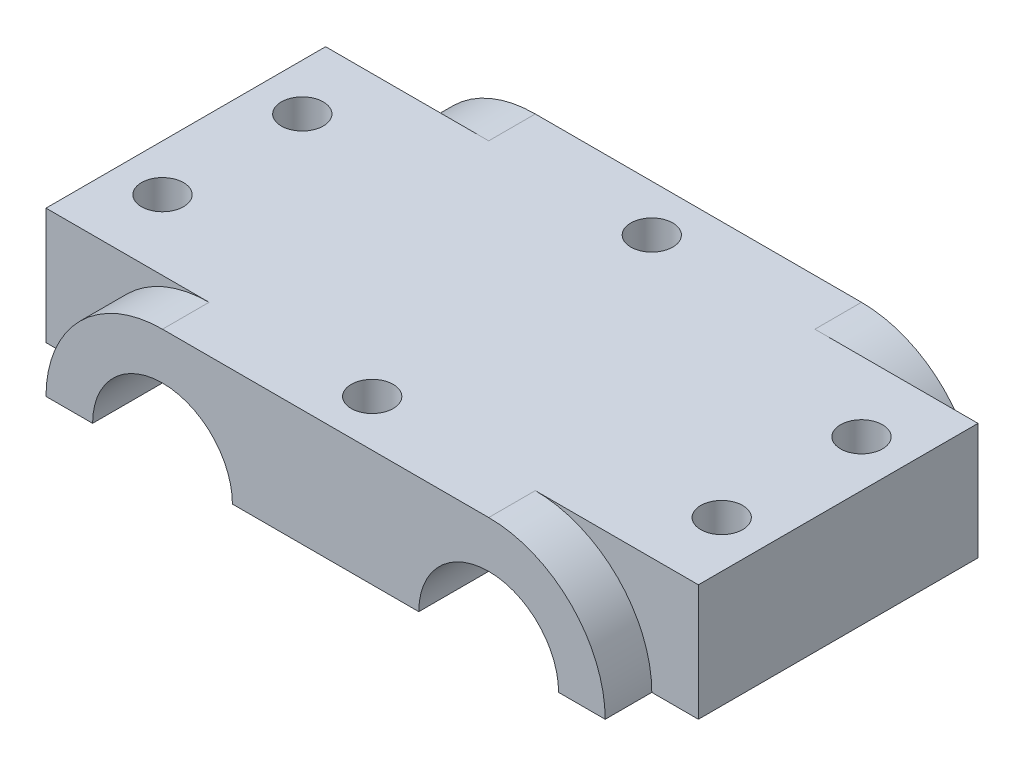
ISO-10303-21;
HEADER;
FILE_DESCRIPTION(('STEP AP214'),'2;1');
FILE_NAME('part.step','',(''),(''),'','','');
FILE_SCHEMA(('AUTOMOTIVE_DESIGN { 1 0 10303 214 1 1 1 1 }'));
ENDSEC;
DATA;
#1=APPLICATION_CONTEXT('core data for automotive mechanical design processes');
#2=APPLICATION_PROTOCOL_DEFINITION('international standard','automotive_design',2000,#1);
#3=PRODUCT_CONTEXT('',#1,'mechanical');
#4=PRODUCT('Part','Part','',(#3));
#5=PRODUCT_RELATED_PRODUCT_CATEGORY('part','',(#4));
#6=PRODUCT_DEFINITION_FORMATION('','',#4);
#7=PRODUCT_DEFINITION_CONTEXT('part definition',#1,'design');
#8=PRODUCT_DEFINITION('design','',#6,#7);
#9=PRODUCT_DEFINITION_SHAPE('','',#8);
#10=(LENGTH_UNIT() NAMED_UNIT(*) SI_UNIT(.MILLI.,.METRE.));
#11=(NAMED_UNIT(*) PLANE_ANGLE_UNIT() SI_UNIT($,.RADIAN.));
#12=(NAMED_UNIT(*) SI_UNIT($,.STERADIAN.) SOLID_ANGLE_UNIT());
#13=UNCERTAINTY_MEASURE_WITH_UNIT(LENGTH_MEASURE(1.E-05),#10,'distance_accuracy_value','');
#14=(GEOMETRIC_REPRESENTATION_CONTEXT(3) GLOBAL_UNCERTAINTY_ASSIGNED_CONTEXT((#13)) GLOBAL_UNIT_ASSIGNED_CONTEXT((#10,
#11,#12)) REPRESENTATION_CONTEXT('',''));
#15=CARTESIAN_POINT('',(0.,0.,0.));
#16=DIRECTION('',(0.,0.,1.));
#17=DIRECTION('',(1.,0.,0.));
#18=AXIS2_PLACEMENT_3D('',#15,#16,#17);
#19=CARTESIAN_POINT('',(35.,-6.25,20.));
#20=DIRECTION('',(0.,1.,0.));
#21=DIRECTION('',(-1.,0.,0.));
#22=AXIS2_PLACEMENT_3D('',#19,#20,#21);
#23=PLANE('',#22);
#24=CARTESIAN_POINT('',(0.,-6.25000000000001,-15.));
#25=DIRECTION('',(0.,1.,0.));
#26=DIRECTION('',(1.,0.,0.));
#27=AXIS2_PLACEMENT_3D('',#24,#25,#26);
#28=CIRCLE('',#27,2.25);
#29=CARTESIAN_POINT('',(2.25,-6.25000000000001,-15.));
#30=VERTEX_POINT('',#29);
#31=EDGE_CURVE('E271',#30,#30,#28,.T.);
#32=ORIENTED_EDGE('',*,*,#31,.T.);
#33=EDGE_LOOP('',(#32));
#34=FACE_BOUND('',#33,.T.);
#35=CARTESIAN_POINT('',(0.,-6.25000000000001,15.));
#36=DIRECTION('',(0.,1.,0.));
#37=DIRECTION('',(-1.,0.,0.));
#38=AXIS2_PLACEMENT_3D('',#35,#36,#37);
#39=CIRCLE('',#38,2.25);
#40=CARTESIAN_POINT('',(-2.24999999999999,-6.25000000000001,15.));
#41=VERTEX_POINT('',#40);
#42=EDGE_CURVE('E281',#41,#41,#39,.T.);
#43=ORIENTED_EDGE('',*,*,#42,.T.);
#44=EDGE_LOOP('',(#43));
#45=FACE_BOUND('',#44,.T.);
#46=DIRECTION('',(1.,0.,0.));
#47=VECTOR('',#46,1.);
#48=CARTESIAN_POINT('',(35.,-6.25,-20.));
#49=LINE('',#48,#47);
#50=CARTESIAN_POINT('',(-10.,-6.25,-20.));
#51=VERTEX_POINT('',#50);
#52=CARTESIAN_POINT('',(10.,-6.25,-20.));
#53=VERTEX_POINT('',#52);
#54=EDGE_CURVE('E158',#51,#53,#49,.T.);
#55=ORIENTED_EDGE('',*,*,#54,.T.);
#56=DIRECTION('',(0.,0.,1.));
#57=VECTOR('',#56,1.);
#58=CARTESIAN_POINT('',(10.,-6.25,-20.));
#59=LINE('',#58,#57);
#60=CARTESIAN_POINT('',(10.,-6.25,20.));
#61=VERTEX_POINT('',#60);
#62=EDGE_CURVE('E12',#53,#61,#59,.T.);
#63=ORIENTED_EDGE('',*,*,#62,.T.);
#64=DIRECTION('',(1.,0.,0.));
#65=VECTOR('',#64,1.);
#66=CARTESIAN_POINT('',(35.,-6.25,20.));
#67=LINE('',#66,#65);
#68=CARTESIAN_POINT('',(-10.,-6.25,20.));
#69=VERTEX_POINT('',#68);
#70=EDGE_CURVE('E177',#69,#61,#67,.T.);
#71=ORIENTED_EDGE('',*,*,#70,.F.);
#72=DIRECTION('',(0.,0.,1.));
#73=VECTOR('',#72,1.);
#74=CARTESIAN_POINT('',(-10.,-6.25,-20.));
#75=LINE('',#74,#73);
#76=EDGE_CURVE('E174',#51,#69,#75,.T.);
#77=ORIENTED_EDGE('',*,*,#76,.F.);
#78=EDGE_LOOP('',(#55,#63,#71,#77));
#79=FACE_BOUND('',#78,.T.);
#80=ADVANCED_FACE('F37',(#34,#45,#79),#23,.F.);
#81=CARTESIAN_POINT('',(35.,-33.75,-15.));
#82=DIRECTION('',(0.,0.,-1.));
#83=DIRECTION('',(-1.,0.,0.));
#84=AXIS2_PLACEMENT_3D('',#81,#82,#83);
#85=PLANE('',#84);
#86=DIRECTION('',(-1.,0.,0.));
#87=VECTOR('',#86,1.);
#88=CARTESIAN_POINT('',(35.,-6.25,-15.));
#89=LINE('',#88,#87);
#90=CARTESIAN_POINT('',(35.,-6.25,-15.));
#91=VERTEX_POINT('',#90);
#92=CARTESIAN_POINT('',(30.,-6.25,-15.));
#93=VERTEX_POINT('',#92);
#94=EDGE_CURVE('E180',#91,#93,#89,.T.);
#95=ORIENTED_EDGE('',*,*,#94,.T.);
#96=CARTESIAN_POINT('',(17.5,-6.25,-15.));
#97=DIRECTION('',(0.,0.,1.));
#98=DIRECTION('',(-1.,0.,0.));
#99=AXIS2_PLACEMENT_3D('',#96,#97,#98);
#100=CIRCLE('',#99,12.5);
#101=CARTESIAN_POINT('',(17.5,6.25,-15.));
#102=VERTEX_POINT('',#101);
#103=EDGE_CURVE('E335',#93,#102,#100,.T.);
#104=ORIENTED_EDGE('',*,*,#103,.T.);
#105=DIRECTION('',(-1.,0.,0.));
#106=VECTOR('',#105,1.);
#107=CARTESIAN_POINT('',(35.,6.25,-15.));
#108=LINE('',#107,#106);
#109=CARTESIAN_POINT('',(35.,6.25,-15.));
#110=VERTEX_POINT('',#109);
#111=EDGE_CURVE('E212',#110,#102,#108,.T.);
#112=ORIENTED_EDGE('',*,*,#111,.F.);
#113=DIRECTION('',(0.,1.,0.));
#114=VECTOR('',#113,1.);
#115=CARTESIAN_POINT('',(35.,-33.75,-15.));
#116=LINE('',#115,#114);
#117=EDGE_CURVE('E64',#91,#110,#116,.T.);
#118=ORIENTED_EDGE('',*,*,#117,.F.);
#119=EDGE_LOOP('',(#95,#104,#112,#118));
#120=FACE_BOUND('',#119,.T.);
#121=ADVANCED_FACE('F332',(#120),#85,.T.);
#122=CARTESIAN_POINT('',(22.5,-33.75,15.));
#123=DIRECTION('',(0.,0.,1.));
#124=DIRECTION('',(1.,0.,0.));
#125=AXIS2_PLACEMENT_3D('',#122,#123,#124);
#126=PLANE('',#125);
#127=CARTESIAN_POINT('',(17.5,-6.25,15.));
#128=DIRECTION('',(0.,0.,1.));
#129=DIRECTION('',(-1.,0.,0.));
#130=AXIS2_PLACEMENT_3D('',#127,#128,#129);
#131=CIRCLE('',#130,12.5);
#132=CARTESIAN_POINT('',(30.,-6.25,15.));
#133=VERTEX_POINT('',#132);
#134=CARTESIAN_POINT('',(17.5,6.25,15.));
#135=VERTEX_POINT('',#134);
#136=EDGE_CURVE('E343',#133,#135,#131,.T.);
#137=ORIENTED_EDGE('',*,*,#136,.F.);
#138=DIRECTION('',(1.,0.,0.));
#139=VECTOR('',#138,1.);
#140=CARTESIAN_POINT('',(35.,-6.25,15.));
#141=LINE('',#140,#139);
#142=CARTESIAN_POINT('',(35.,-6.25,15.));
#143=VERTEX_POINT('',#142);
#144=EDGE_CURVE('E181',#133,#143,#141,.T.);
#145=ORIENTED_EDGE('',*,*,#144,.T.);
#146=DIRECTION('',(0.,1.,0.));
#147=VECTOR('',#146,1.);
#148=CARTESIAN_POINT('',(35.,-33.75,15.));
#149=LINE('',#148,#147);
#150=CARTESIAN_POINT('',(35.,6.25,15.));
#151=VERTEX_POINT('',#150);
#152=EDGE_CURVE('E214',#143,#151,#149,.T.);
#153=ORIENTED_EDGE('',*,*,#152,.T.);
#154=DIRECTION('',(1.,0.,0.));
#155=VECTOR('',#154,1.);
#156=CARTESIAN_POINT('',(22.5,6.25,15.));
#157=LINE('',#156,#155);
#158=EDGE_CURVE('E213',#135,#151,#157,.T.);
#159=ORIENTED_EDGE('',*,*,#158,.F.);
#160=EDGE_LOOP('',(#137,#145,#153,#159));
#161=FACE_BOUND('',#160,.T.);
#162=ADVANCED_FACE('F317',(#161),#126,.T.);
#163=CARTESIAN_POINT('',(30.,-6.25000000000001,-7.50000000000001));
#164=DIRECTION('',(0.,1.,0.));
#165=DIRECTION('',(-1.,0.,0.));
#166=AXIS2_PLACEMENT_3D('',#163,#164,#165);
#167=CYLINDRICAL_SURFACE('',#166,2.25);
#168=CARTESIAN_POINT('',(30.,6.25,-7.50000000000001));
#169=DIRECTION('',(0.,1.,0.));
#170=DIRECTION('',(1.,0.,0.));
#171=AXIS2_PLACEMENT_3D('',#168,#169,#170);
#172=CIRCLE('',#171,2.25);
#173=CARTESIAN_POINT('',(32.25,6.25,-7.50000000000001));
#174=VERTEX_POINT('',#173);
#175=EDGE_CURVE('E274',#174,#174,#172,.T.);
#176=ORIENTED_EDGE('',*,*,#175,.T.);
#177=EDGE_LOOP('',(#176));
#178=FACE_BOUND('',#177,.T.);
#179=CARTESIAN_POINT('',(30.,-6.25000000000001,-7.50000000000001));
#180=DIRECTION('',(0.,1.,0.));
#181=DIRECTION('',(1.,0.,0.));
#182=AXIS2_PLACEMENT_3D('',#179,#180,#181);
#183=CIRCLE('',#182,2.25);
#184=CARTESIAN_POINT('',(32.25,-6.25000000000001,-7.50000000000001));
#185=VERTEX_POINT('',#184);
#186=EDGE_CURVE('E279',#185,#185,#183,.T.);
#187=ORIENTED_EDGE('',*,*,#186,.F.);
#188=EDGE_LOOP('',(#187));
#189=FACE_BOUND('',#188,.T.);
#190=ADVANCED_FACE('F402',(#178,#189),#167,.F.);
#191=CARTESIAN_POINT('',(30.,-6.25000000000001,7.49999999999999));
#192=DIRECTION('',(0.,1.,0.));
#193=DIRECTION('',(-1.,0.,0.));
#194=AXIS2_PLACEMENT_3D('',#191,#192,#193);
#195=CYLINDRICAL_SURFACE('',#194,2.25);
#196=CARTESIAN_POINT('',(30.,6.25,7.49999999999999));
#197=DIRECTION('',(0.,1.,0.));
#198=DIRECTION('',(1.,0.,0.));
#199=AXIS2_PLACEMENT_3D('',#196,#197,#198);
#200=CIRCLE('',#199,2.25);
#201=CARTESIAN_POINT('',(32.25,6.25,7.49999999999999));
#202=VERTEX_POINT('',#201);
#203=EDGE_CURVE('E294',#202,#202,#200,.T.);
#204=ORIENTED_EDGE('',*,*,#203,.T.);
#205=EDGE_LOOP('',(#204));
#206=FACE_BOUND('',#205,.T.);
#207=CARTESIAN_POINT('',(30.,-6.25000000000001,7.49999999999999));
#208=DIRECTION('',(0.,1.,0.));
#209=DIRECTION('',(1.,0.,0.));
#210=AXIS2_PLACEMENT_3D('',#207,#208,#209);
#211=CIRCLE('',#210,2.25);
#212=CARTESIAN_POINT('',(32.25,-6.25000000000001,7.49999999999999));
#213=VERTEX_POINT('',#212);
#214=EDGE_CURVE('E280',#213,#213,#211,.T.);
#215=ORIENTED_EDGE('',*,*,#214,.F.);
#216=EDGE_LOOP('',(#215));
#217=FACE_BOUND('',#216,.T.);
#218=ADVANCED_FACE('F396',(#206,#217),#195,.F.);
#219=CARTESIAN_POINT('',(35.,6.25,20.));
#220=DIRECTION('',(0.,-1.,0.));
#221=DIRECTION('',(1.,0.,0.));
#222=AXIS2_PLACEMENT_3D('',#219,#220,#221);
#223=PLANE('',#222);
#224=CARTESIAN_POINT('',(0.,6.25,-15.));
#225=DIRECTION('',(0.,1.,0.));
#226=DIRECTION('',(1.,0.,0.));
#227=AXIS2_PLACEMENT_3D('',#224,#225,#226);
#228=CIRCLE('',#227,2.25);
#229=CARTESIAN_POINT('',(2.25,6.25,-15.));
#230=VERTEX_POINT('',#229);
#231=EDGE_CURVE('E290',#230,#230,#228,.T.);
#232=ORIENTED_EDGE('',*,*,#231,.F.);
#233=EDGE_LOOP('',(#232));
#234=FACE_BOUND('',#233,.T.);
#235=CARTESIAN_POINT('',(0.,6.25,15.));
#236=DIRECTION('',(0.,1.,0.));
#237=DIRECTION('',(-1.,0.,0.));
#238=AXIS2_PLACEMENT_3D('',#235,#236,#237);
#239=CIRCLE('',#238,2.25);
#240=CARTESIAN_POINT('',(-2.25,6.25,15.));
#241=VERTEX_POINT('',#240);
#242=EDGE_CURVE('E282',#241,#241,#239,.T.);
#243=ORIENTED_EDGE('',*,*,#242,.F.);
#244=EDGE_LOOP('',(#243));
#245=FACE_BOUND('',#244,.T.);
#246=CARTESIAN_POINT('',(-30.,6.25,-7.5));
#247=DIRECTION('',(0.,1.,0.));
#248=DIRECTION('',(-1.,0.,0.));
#249=AXIS2_PLACEMENT_3D('',#246,#247,#248);
#250=CIRCLE('',#249,2.25);
#251=CARTESIAN_POINT('',(-32.25,6.25,-7.5));
#252=VERTEX_POINT('',#251);
#253=EDGE_CURVE('E293',#252,#252,#250,.T.);
#254=ORIENTED_EDGE('',*,*,#253,.F.);
#255=EDGE_LOOP('',(#254));
#256=FACE_BOUND('',#255,.T.);
#257=CARTESIAN_POINT('',(-30.,6.25,7.5));
#258=DIRECTION('',(0.,1.,0.));
#259=DIRECTION('',(-1.,0.,0.));
#260=AXIS2_PLACEMENT_3D('',#257,#258,#259);
#261=CIRCLE('',#260,2.25);
#262=CARTESIAN_POINT('',(-32.25,6.25,7.5));
#263=VERTEX_POINT('',#262);
#264=EDGE_CURVE('E289',#263,#263,#261,.T.);
#265=ORIENTED_EDGE('',*,*,#264,.F.);
#266=EDGE_LOOP('',(#265));
#267=FACE_BOUND('',#266,.T.);
#268=DIRECTION('',(0.,0.,1.));
#269=VECTOR('',#268,1.);
#270=CARTESIAN_POINT('',(17.5,6.25,15.));
#271=LINE('',#270,#269);
#272=CARTESIAN_POINT('',(17.5,6.25,20.));
#273=VERTEX_POINT('',#272);
#274=EDGE_CURVE('E248',#135,#273,#271,.T.);
#275=ORIENTED_EDGE('',*,*,#274,.F.);
#276=ORIENTED_EDGE('',*,*,#158,.T.);
#277=DIRECTION('',(0.,0.,-1.));
#278=VECTOR('',#277,1.);
#279=CARTESIAN_POINT('',(35.,6.25,20.));
#280=LINE('',#279,#278);
#281=EDGE_CURVE('E188',#151,#110,#280,.T.);
#282=ORIENTED_EDGE('',*,*,#281,.T.);
#283=ORIENTED_EDGE('',*,*,#111,.T.);
#284=DIRECTION('',(0.,0.,-1.));
#285=VECTOR('',#284,1.);
#286=CARTESIAN_POINT('',(17.5,6.25,-15.));
#287=LINE('',#286,#285);
#288=CARTESIAN_POINT('',(17.5,6.25,-20.));
#289=VERTEX_POINT('',#288);
#290=EDGE_CURVE('E333',#102,#289,#287,.T.);
#291=ORIENTED_EDGE('',*,*,#290,.T.);
#292=DIRECTION('',(-1.,0.,0.));
#293=VECTOR('',#292,1.);
#294=CARTESIAN_POINT('',(35.,6.25,-20.));
#295=LINE('',#294,#293);
#296=CARTESIAN_POINT('',(-17.5,6.25,-20.));
#297=VERTEX_POINT('',#296);
#298=EDGE_CURVE('E176',#289,#297,#295,.T.);
#299=ORIENTED_EDGE('',*,*,#298,.T.);
#300=DIRECTION('',(0.,0.,-1.));
#301=VECTOR('',#300,1.);
#302=CARTESIAN_POINT('',(-17.5,6.25,-15.));
#303=LINE('',#302,#301);
#304=CARTESIAN_POINT('',(-17.5,6.25,-15.));
#305=VERTEX_POINT('',#304);
#306=EDGE_CURVE('E244',#305,#297,#303,.T.);
#307=ORIENTED_EDGE('',*,*,#306,.F.);
#308=DIRECTION('',(-1.,0.,0.));
#309=VECTOR('',#308,1.);
#310=CARTESIAN_POINT('',(-22.5,6.25,-15.));
#311=LINE('',#310,#309);
#312=CARTESIAN_POINT('',(-35.,6.25,-15.));
#313=VERTEX_POINT('',#312);
#314=EDGE_CURVE('E310',#305,#313,#311,.T.);
#315=ORIENTED_EDGE('',*,*,#314,.T.);
#316=DIRECTION('',(0.,0.,-1.));
#317=VECTOR('',#316,1.);
#318=CARTESIAN_POINT('',(-35.,6.25,20.));
#319=LINE('',#318,#317);
#320=CARTESIAN_POINT('',(-35.,6.25,15.));
#321=VERTEX_POINT('',#320);
#322=EDGE_CURVE('E190',#321,#313,#319,.T.);
#323=ORIENTED_EDGE('',*,*,#322,.F.);
#324=DIRECTION('',(1.,0.,0.));
#325=VECTOR('',#324,1.);
#326=CARTESIAN_POINT('',(-35.,6.25,15.));
#327=LINE('',#326,#325);
#328=CARTESIAN_POINT('',(-17.5,6.25,15.));
#329=VERTEX_POINT('',#328);
#330=EDGE_CURVE('E242',#321,#329,#327,.T.);
#331=ORIENTED_EDGE('',*,*,#330,.T.);
#332=DIRECTION('',(0.,0.,1.));
#333=VECTOR('',#332,1.);
#334=CARTESIAN_POINT('',(-17.5,6.25,15.));
#335=LINE('',#334,#333);
#336=CARTESIAN_POINT('',(-17.5,6.25,20.));
#337=VERTEX_POINT('',#336);
#338=EDGE_CURVE('E240',#329,#337,#335,.T.);
#339=ORIENTED_EDGE('',*,*,#338,.T.);
#340=DIRECTION('',(-1.,0.,0.));
#341=VECTOR('',#340,1.);
#342=CARTESIAN_POINT('',(35.,6.25,20.));
#343=LINE('',#342,#341);
#344=EDGE_CURVE('E183',#273,#337,#343,.T.);
#345=ORIENTED_EDGE('',*,*,#344,.F.);
#346=EDGE_LOOP('',(#275,#276,#282,#283,#291,#299,#307,#315,#323,#331,#339,#345));
#347=FACE_BOUND('',#346,.T.);
#348=ORIENTED_EDGE('',*,*,#175,.F.);
#349=EDGE_LOOP('',(#348));
#350=FACE_BOUND('',#349,.T.);
#351=ORIENTED_EDGE('',*,*,#203,.F.);
#352=EDGE_LOOP('',(#351));
#353=FACE_BOUND('',#352,.T.);
#354=ADVANCED_FACE('F245',(#234,#245,#256,#267,#347,#350,#353),#223,.F.);
#355=CARTESIAN_POINT('',(0.,0.,20.));
#356=DIRECTION('',(0.,0.,1.));
#357=DIRECTION('',(1.,0.,0.));
#358=AXIS2_PLACEMENT_3D('',#355,#356,#357);
#359=PLANE('',#358);
#360=ORIENTED_EDGE('',*,*,#70,.T.);
#361=CARTESIAN_POINT('',(17.5,-6.25,20.));
#362=DIRECTION('',(0.,0.,1.));
#363=DIRECTION('',(-1.,0.,0.));
#364=AXIS2_PLACEMENT_3D('',#361,#362,#363);
#365=CIRCLE('',#364,7.5);
#366=CARTESIAN_POINT('',(25.,-6.25,20.));
#367=VERTEX_POINT('',#366);
#368=EDGE_CURVE('E169',#367,#61,#365,.T.);
#369=ORIENTED_EDGE('',*,*,#368,.F.);
#370=DIRECTION('',(-1.,0.,0.));
#371=VECTOR('',#370,1.);
#372=CARTESIAN_POINT('',(30.,-6.25,20.));
#373=LINE('',#372,#371);
#374=CARTESIAN_POINT('',(30.,-6.25,20.));
#375=VERTEX_POINT('',#374);
#376=EDGE_CURVE('E164',#375,#367,#373,.T.);
#377=ORIENTED_EDGE('',*,*,#376,.F.);
#378=CARTESIAN_POINT('',(17.5,-6.25,20.));
#379=DIRECTION('',(0.,0.,1.));
#380=DIRECTION('',(-1.,0.,0.));
#381=AXIS2_PLACEMENT_3D('',#378,#379,#380);
#382=CIRCLE('',#381,12.5);
#383=EDGE_CURVE('E229',#375,#273,#382,.T.);
#384=ORIENTED_EDGE('',*,*,#383,.T.);
#385=ORIENTED_EDGE('',*,*,#344,.T.);
#386=CARTESIAN_POINT('',(-17.5,-6.25,20.));
#387=DIRECTION('',(0.,0.,1.));
#388=DIRECTION('',(1.,0.,0.));
#389=AXIS2_PLACEMENT_3D('',#386,#387,#388);
#390=CIRCLE('',#389,12.5);
#391=CARTESIAN_POINT('',(-30.,-6.25,20.));
#392=VERTEX_POINT('',#391);
#393=EDGE_CURVE('E227',#337,#392,#390,.T.);
#394=ORIENTED_EDGE('',*,*,#393,.T.);
#395=DIRECTION('',(1.,0.,0.));
#396=VECTOR('',#395,1.);
#397=CARTESIAN_POINT('',(-30.,-6.25,20.));
#398=LINE('',#397,#396);
#399=CARTESIAN_POINT('',(-25.,-6.25,20.));
#400=VERTEX_POINT('',#399);
#401=EDGE_CURVE('E239',#392,#400,#398,.T.);
#402=ORIENTED_EDGE('',*,*,#401,.T.);
#403=CARTESIAN_POINT('',(-17.5,-6.25,20.));
#404=DIRECTION('',(0.,0.,-1.));
#405=DIRECTION('',(1.,0.,0.));
#406=AXIS2_PLACEMENT_3D('',#403,#404,#405);
#407=CIRCLE('',#406,7.5);
#408=EDGE_CURVE('E257',#400,#69,#407,.T.);
#409=ORIENTED_EDGE('',*,*,#408,.T.);
#410=EDGE_LOOP('',(#360,#369,#377,#384,#385,#394,#402,#409));
#411=FACE_BOUND('',#410,.T.);
#412=ADVANCED_FACE('F223',(#411),#359,.T.);
#413=CARTESIAN_POINT('',(0.,0.,-20.));
#414=DIRECTION('',(0.,0.,1.));
#415=DIRECTION('',(1.,0.,0.));
#416=AXIS2_PLACEMENT_3D('',#413,#414,#415);
#417=PLANE('',#416);
#418=CARTESIAN_POINT('',(17.5,-6.25,-20.));
#419=DIRECTION('',(0.,0.,1.));
#420=DIRECTION('',(-1.,0.,0.));
#421=AXIS2_PLACEMENT_3D('',#418,#419,#420);
#422=CIRCLE('',#421,7.5);
#423=CARTESIAN_POINT('',(25.,-6.25,-20.));
#424=VERTEX_POINT('',#423);
#425=EDGE_CURVE('E153',#424,#53,#422,.T.);
#426=ORIENTED_EDGE('',*,*,#425,.T.);
#427=ORIENTED_EDGE('',*,*,#54,.F.);
#428=CARTESIAN_POINT('',(-17.5,-6.25,-20.));
#429=DIRECTION('',(0.,0.,-1.));
#430=DIRECTION('',(1.,0.,0.));
#431=AXIS2_PLACEMENT_3D('',#428,#429,#430);
#432=CIRCLE('',#431,7.5);
#433=CARTESIAN_POINT('',(-25.,-6.25,-20.));
#434=VERTEX_POINT('',#433);
#435=EDGE_CURVE('E256',#434,#51,#432,.T.);
#436=ORIENTED_EDGE('',*,*,#435,.F.);
#437=DIRECTION('',(1.,0.,0.));
#438=VECTOR('',#437,1.);
#439=CARTESIAN_POINT('',(-30.,-6.25,-20.));
#440=LINE('',#439,#438);
#441=CARTESIAN_POINT('',(-30.,-6.25,-20.));
#442=VERTEX_POINT('',#441);
#443=EDGE_CURVE('E253',#442,#434,#440,.T.);
#444=ORIENTED_EDGE('',*,*,#443,.F.);
#445=CARTESIAN_POINT('',(-17.5,-6.25,-20.));
#446=DIRECTION('',(0.,0.,1.));
#447=DIRECTION('',(1.,0.,0.));
#448=AXIS2_PLACEMENT_3D('',#445,#446,#447);
#449=CIRCLE('',#448,12.5);
#450=EDGE_CURVE('E254',#297,#442,#449,.T.);
#451=ORIENTED_EDGE('',*,*,#450,.F.);
#452=ORIENTED_EDGE('',*,*,#298,.F.);
#453=CARTESIAN_POINT('',(17.5,-6.25,-20.));
#454=DIRECTION('',(0.,0.,1.));
#455=DIRECTION('',(-1.,0.,0.));
#456=AXIS2_PLACEMENT_3D('',#453,#454,#455);
#457=CIRCLE('',#456,12.5);
#458=CARTESIAN_POINT('',(30.,-6.25,-20.));
#459=VERTEX_POINT('',#458);
#460=EDGE_CURVE('E337',#459,#289,#457,.T.);
#461=ORIENTED_EDGE('',*,*,#460,.F.);
#462=DIRECTION('',(-1.,0.,0.));
#463=VECTOR('',#462,1.);
#464=CARTESIAN_POINT('',(30.,-6.25,-20.));
#465=LINE('',#464,#463);
#466=EDGE_CURVE('E162',#459,#424,#465,.T.);
#467=ORIENTED_EDGE('',*,*,#466,.T.);
#468=EDGE_LOOP('',(#426,#427,#436,#444,#451,#452,#461,#467));
#469=FACE_BOUND('',#468,.T.);
#470=ADVANCED_FACE('F160',(#469),#417,.F.);
#471=CARTESIAN_POINT('',(-30.,-6.25000000000001,7.5));
#472=DIRECTION('',(0.,1.,0.));
#473=DIRECTION('',(-1.,0.,0.));
#474=AXIS2_PLACEMENT_3D('',#471,#472,#473);
#475=CIRCLE('',#474,2.25);
#476=CARTESIAN_POINT('',(-32.25,-6.25000000000001,7.5));
#477=VERTEX_POINT('',#476);
#478=EDGE_CURVE('E292',#477,#477,#475,.T.);
#479=ORIENTED_EDGE('',*,*,#478,.T.);
#480=EDGE_LOOP('',(#479));
#481=FACE_BOUND('',#480,.T.);
#482=CARTESIAN_POINT('',(-30.,-6.25000000000001,-7.5));
#483=DIRECTION('',(0.,1.,0.));
#484=DIRECTION('',(-1.,0.,0.));
#485=AXIS2_PLACEMENT_3D('',#482,#483,#484);
#486=CIRCLE('',#485,2.25);
#487=CARTESIAN_POINT('',(-32.25,-6.25000000000001,-7.5));
#488=VERTEX_POINT('',#487);
#489=EDGE_CURVE('E302',#488,#488,#486,.T.);
#490=ORIENTED_EDGE('',*,*,#489,.T.);
#491=EDGE_LOOP('',(#490));
#492=FACE_BOUND('',#491,.T.);
#493=DIRECTION('',(0.,0.,1.));
#494=VECTOR('',#493,1.);
#495=CARTESIAN_POINT('',(-25.,-6.25,-20.));
#496=LINE('',#495,#494);
#497=EDGE_CURVE('E265',#434,#400,#496,.T.);
#498=ORIENTED_EDGE('',*,*,#497,.T.);
#499=ORIENTED_EDGE('',*,*,#401,.F.);
#500=DIRECTION('',(0.,0.,1.));
#501=VECTOR('',#500,1.);
#502=CARTESIAN_POINT('',(-30.,-6.25,-20.));
#503=LINE('',#502,#501);
#504=CARTESIAN_POINT('',(-30.,-6.25000000000001,15.));
#505=VERTEX_POINT('',#504);
#506=EDGE_CURVE('E238',#505,#392,#503,.T.);
#507=ORIENTED_EDGE('',*,*,#506,.F.);
#508=DIRECTION('',(1.,0.,0.));
#509=VECTOR('',#508,1.);
#510=CARTESIAN_POINT('',(35.,-6.25,15.));
#511=LINE('',#510,#509);
#512=CARTESIAN_POINT('',(-35.,-6.25000000000001,15.));
#513=VERTEX_POINT('',#512);
#514=EDGE_CURVE('E54',#513,#505,#511,.T.);
#515=ORIENTED_EDGE('',*,*,#514,.F.);
#516=DIRECTION('',(0.,0.,-1.));
#517=VECTOR('',#516,1.);
#518=CARTESIAN_POINT('',(-35.,-6.25000000000001,20.));
#519=LINE('',#518,#517);
#520=CARTESIAN_POINT('',(-35.,-6.25000000000001,-15.));
#521=VERTEX_POINT('',#520);
#522=EDGE_CURVE('E48',#513,#521,#519,.T.);
#523=ORIENTED_EDGE('',*,*,#522,.T.);
#524=DIRECTION('',(-1.,0.,0.));
#525=VECTOR('',#524,1.);
#526=CARTESIAN_POINT('',(35.,-6.25,-15.));
#527=LINE('',#526,#525);
#528=CARTESIAN_POINT('',(-30.,-6.25,-15.));
#529=VERTEX_POINT('',#528);
#530=EDGE_CURVE('E198',#529,#521,#527,.T.);
#531=ORIENTED_EDGE('',*,*,#530,.F.);
#532=EDGE_CURVE('E267',#442,#529,#503,.T.);
#533=ORIENTED_EDGE('',*,*,#532,.F.);
#534=ORIENTED_EDGE('',*,*,#443,.T.);
#535=EDGE_LOOP('',(#498,#499,#507,#515,#523,#531,#533,#534));
#536=FACE_BOUND('',#535,.T.);
#537=ADVANCED_FACE('F200',(#481,#492,#536),#23,.F.);
#538=CARTESIAN_POINT('',(-22.5,-33.75,-15.));
#539=DIRECTION('',(0.,0.,-1.));
#540=DIRECTION('',(-1.,0.,0.));
#541=AXIS2_PLACEMENT_3D('',#538,#539,#540);
#542=PLANE('',#541);
#543=CARTESIAN_POINT('',(-17.5,-6.25,-15.));
#544=DIRECTION('',(0.,0.,-1.));
#545=DIRECTION('',(-1.,0.,0.));
#546=AXIS2_PLACEMENT_3D('',#543,#544,#545);
#547=CIRCLE('',#546,12.5);
#548=EDGE_CURVE('E268',#529,#305,#547,.T.);
#549=ORIENTED_EDGE('',*,*,#548,.F.);
#550=ORIENTED_EDGE('',*,*,#530,.T.);
#551=DIRECTION('',(0.,1.,0.));
#552=VECTOR('',#551,1.);
#553=CARTESIAN_POINT('',(-35.,-33.75,-15.));
#554=LINE('',#553,#552);
#555=EDGE_CURVE('E206',#521,#313,#554,.T.);
#556=ORIENTED_EDGE('',*,*,#555,.T.);
#557=ORIENTED_EDGE('',*,*,#314,.F.);
#558=EDGE_LOOP('',(#549,#550,#556,#557));
#559=FACE_BOUND('',#558,.T.);
#560=ADVANCED_FACE('F363',(#559),#542,.T.);
#561=CARTESIAN_POINT('',(-35.,-33.75,15.));
#562=DIRECTION('',(0.,0.,1.));
#563=DIRECTION('',(1.,0.,0.));
#564=AXIS2_PLACEMENT_3D('',#561,#562,#563);
#565=PLANE('',#564);
#566=CARTESIAN_POINT('',(-17.5,-6.25,15.));
#567=DIRECTION('',(0.,0.,1.));
#568=DIRECTION('',(1.,0.,0.));
#569=AXIS2_PLACEMENT_3D('',#566,#567,#568);
#570=CIRCLE('',#569,12.5);
#571=EDGE_CURVE('E263',#329,#505,#570,.T.);
#572=ORIENTED_EDGE('',*,*,#571,.F.);
#573=ORIENTED_EDGE('',*,*,#330,.F.);
#574=DIRECTION('',(0.,1.,0.));
#575=VECTOR('',#574,1.);
#576=CARTESIAN_POINT('',(-35.,-33.75,15.));
#577=LINE('',#576,#575);
#578=EDGE_CURVE('E207',#513,#321,#577,.T.);
#579=ORIENTED_EDGE('',*,*,#578,.F.);
#580=ORIENTED_EDGE('',*,*,#514,.T.);
#581=EDGE_LOOP('',(#572,#573,#579,#580));
#582=FACE_BOUND('',#581,.T.);
#583=ADVANCED_FACE('F391',(#582),#565,.T.);
#584=CARTESIAN_POINT('',(-35.,-6.25000000000001,20.));
#585=DIRECTION('',(1.,0.,0.));
#586=DIRECTION('',(0.,0.,-1.));
#587=AXIS2_PLACEMENT_3D('',#584,#585,#586);
#588=PLANE('',#587);
#589=ORIENTED_EDGE('',*,*,#578,.T.);
#590=ORIENTED_EDGE('',*,*,#322,.T.);
#591=ORIENTED_EDGE('',*,*,#555,.F.);
#592=ORIENTED_EDGE('',*,*,#522,.F.);
#593=EDGE_LOOP('',(#589,#590,#591,#592));
#594=FACE_BOUND('',#593,.T.);
#595=ADVANCED_FACE('F45',(#594),#588,.F.);
#596=ORIENTED_EDGE('',*,*,#186,.T.);
#597=EDGE_LOOP('',(#596));
#598=FACE_BOUND('',#597,.T.);
#599=ORIENTED_EDGE('',*,*,#214,.T.);
#600=EDGE_LOOP('',(#599));
#601=FACE_BOUND('',#600,.T.);
#602=ORIENTED_EDGE('',*,*,#376,.T.);
#603=DIRECTION('',(0.,0.,1.));
#604=VECTOR('',#603,1.);
#605=CARTESIAN_POINT('',(25.,-6.25,-20.));
#606=LINE('',#605,#604);
#607=EDGE_CURVE('E345',#424,#367,#606,.T.);
#608=ORIENTED_EDGE('',*,*,#607,.F.);
#609=ORIENTED_EDGE('',*,*,#466,.F.);
#610=DIRECTION('',(0.,0.,1.));
#611=VECTOR('',#610,1.);
#612=CARTESIAN_POINT('',(30.,-6.25,-20.));
#613=LINE('',#612,#611);
#614=EDGE_CURVE('E326',#459,#93,#613,.T.);
#615=ORIENTED_EDGE('',*,*,#614,.T.);
#616=ORIENTED_EDGE('',*,*,#94,.F.);
#617=DIRECTION('',(0.,0.,-1.));
#618=VECTOR('',#617,1.);
#619=CARTESIAN_POINT('',(35.,-6.25,20.));
#620=LINE('',#619,#618);
#621=EDGE_CURVE('E194',#143,#91,#620,.T.);
#622=ORIENTED_EDGE('',*,*,#621,.F.);
#623=ORIENTED_EDGE('',*,*,#144,.F.);
#624=EDGE_CURVE('E348',#133,#375,#613,.T.);
#625=ORIENTED_EDGE('',*,*,#624,.T.);
#626=EDGE_LOOP('',(#602,#608,#609,#615,#616,#622,#623,#625));
#627=FACE_BOUND('',#626,.T.);
#628=ADVANCED_FACE('F323',(#598,#601,#627),#23,.F.);
#629=CARTESIAN_POINT('',(35.,-6.25,20.));
#630=DIRECTION('',(-1.,0.,0.));
#631=DIRECTION('',(0.,0.,1.));
#632=AXIS2_PLACEMENT_3D('',#629,#630,#631);
#633=PLANE('',#632);
#634=ORIENTED_EDGE('',*,*,#117,.T.);
#635=ORIENTED_EDGE('',*,*,#281,.F.);
#636=ORIENTED_EDGE('',*,*,#152,.F.);
#637=ORIENTED_EDGE('',*,*,#621,.T.);
#638=EDGE_LOOP('',(#634,#635,#636,#637));
#639=FACE_BOUND('',#638,.T.);
#640=ADVANCED_FACE('F325',(#639),#633,.F.);
#641=CARTESIAN_POINT('',(-30.,-6.25000000000001,-7.5));
#642=DIRECTION('',(0.,1.,0.));
#643=DIRECTION('',(-1.,0.,0.));
#644=AXIS2_PLACEMENT_3D('',#641,#642,#643);
#645=CYLINDRICAL_SURFACE('',#644,2.25);
#646=ORIENTED_EDGE('',*,*,#489,.F.);
#647=EDGE_LOOP('',(#646));
#648=FACE_BOUND('',#647,.T.);
#649=ORIENTED_EDGE('',*,*,#253,.T.);
#650=EDGE_LOOP('',(#649));
#651=FACE_BOUND('',#650,.T.);
#652=ADVANCED_FACE('F394',(#648,#651),#645,.F.);
#653=CARTESIAN_POINT('',(0.,-6.25000000000001,15.));
#654=DIRECTION('',(0.,1.,0.));
#655=DIRECTION('',(-1.,0.,0.));
#656=AXIS2_PLACEMENT_3D('',#653,#654,#655);
#657=CYLINDRICAL_SURFACE('',#656,2.25);
#658=ORIENTED_EDGE('',*,*,#42,.F.);
#659=EDGE_LOOP('',(#658));
#660=FACE_BOUND('',#659,.T.);
#661=ORIENTED_EDGE('',*,*,#242,.T.);
#662=EDGE_LOOP('',(#661));
#663=FACE_BOUND('',#662,.T.);
#664=ADVANCED_FACE('F416',(#660,#663),#657,.F.);
#665=CARTESIAN_POINT('',(-30.,-6.25000000000001,7.5));
#666=DIRECTION('',(0.,1.,0.));
#667=DIRECTION('',(-1.,0.,0.));
#668=AXIS2_PLACEMENT_3D('',#665,#666,#667);
#669=CYLINDRICAL_SURFACE('',#668,2.25);
#670=ORIENTED_EDGE('',*,*,#478,.F.);
#671=EDGE_LOOP('',(#670));
#672=FACE_BOUND('',#671,.T.);
#673=ORIENTED_EDGE('',*,*,#264,.T.);
#674=EDGE_LOOP('',(#673));
#675=FACE_BOUND('',#674,.T.);
#676=ADVANCED_FACE('F411',(#672,#675),#669,.F.);
#677=CARTESIAN_POINT('',(0.,-6.25000000000001,-15.));
#678=DIRECTION('',(0.,1.,0.));
#679=DIRECTION('',(-1.,0.,0.));
#680=AXIS2_PLACEMENT_3D('',#677,#678,#679);
#681=CYLINDRICAL_SURFACE('',#680,2.25);
#682=ORIENTED_EDGE('',*,*,#31,.F.);
#683=EDGE_LOOP('',(#682));
#684=FACE_BOUND('',#683,.T.);
#685=ORIENTED_EDGE('',*,*,#231,.T.);
#686=EDGE_LOOP('',(#685));
#687=FACE_BOUND('',#686,.T.);
#688=ADVANCED_FACE('F372',(#684,#687),#681,.F.);
#689=CARTESIAN_POINT('',(-17.5,-6.25,-20.));
#690=DIRECTION('',(0.,0.,1.));
#691=DIRECTION('',(1.,0.,0.));
#692=AXIS2_PLACEMENT_3D('',#689,#690,#691);
#693=CYLINDRICAL_SURFACE('',#692,12.5);
#694=ORIENTED_EDGE('',*,*,#393,.F.);
#695=ORIENTED_EDGE('',*,*,#338,.F.);
#696=ORIENTED_EDGE('',*,*,#571,.T.);
#697=ORIENTED_EDGE('',*,*,#506,.T.);
#698=EDGE_LOOP('',(#694,#695,#696,#697));
#699=FACE_BOUND('',#698,.T.);
#700=ADVANCED_FACE('F236',(#699),#693,.T.);
#701=CARTESIAN_POINT('',(-17.5,-6.25,-20.));
#702=DIRECTION('',(0.,0.,1.));
#703=DIRECTION('',(1.,0.,0.));
#704=AXIS2_PLACEMENT_3D('',#701,#702,#703);
#705=CYLINDRICAL_SURFACE('',#704,7.5);
#706=ORIENTED_EDGE('',*,*,#408,.F.);
#707=ORIENTED_EDGE('',*,*,#497,.F.);
#708=ORIENTED_EDGE('',*,*,#435,.T.);
#709=ORIENTED_EDGE('',*,*,#76,.T.);
#710=EDGE_LOOP('',(#706,#707,#708,#709));
#711=FACE_BOUND('',#710,.T.);
#712=ADVANCED_FACE('F364',(#711),#705,.F.);
#713=ORIENTED_EDGE('',*,*,#548,.T.);
#714=ORIENTED_EDGE('',*,*,#306,.T.);
#715=ORIENTED_EDGE('',*,*,#450,.T.);
#716=ORIENTED_EDGE('',*,*,#532,.T.);
#717=EDGE_LOOP('',(#713,#714,#715,#716));
#718=FACE_BOUND('',#717,.T.);
#719=ADVANCED_FACE('F359',(#718),#693,.T.);
#720=CARTESIAN_POINT('',(17.5,-6.25,15.));
#721=DIRECTION('',(0.,0.,1.));
#722=DIRECTION('',(1.,0.,0.));
#723=AXIS2_PLACEMENT_3D('',#720,#721,#722);
#724=CYLINDRICAL_SURFACE('',#723,12.5);
#725=ORIENTED_EDGE('',*,*,#383,.F.);
#726=ORIENTED_EDGE('',*,*,#624,.F.);
#727=ORIENTED_EDGE('',*,*,#136,.T.);
#728=ORIENTED_EDGE('',*,*,#274,.T.);
#729=EDGE_LOOP('',(#725,#726,#727,#728));
#730=FACE_BOUND('',#729,.T.);
#731=ADVANCED_FACE('F350',(#730),#724,.T.);
#732=CARTESIAN_POINT('',(17.5,-6.25,-15.));
#733=DIRECTION('',(0.,0.,-1.));
#734=DIRECTION('',(-1.,0.,0.));
#735=AXIS2_PLACEMENT_3D('',#732,#733,#734);
#736=CYLINDRICAL_SURFACE('',#735,12.5);
#737=ORIENTED_EDGE('',*,*,#460,.T.);
#738=ORIENTED_EDGE('',*,*,#290,.F.);
#739=ORIENTED_EDGE('',*,*,#103,.F.);
#740=ORIENTED_EDGE('',*,*,#614,.F.);
#741=EDGE_LOOP('',(#737,#738,#739,#740));
#742=FACE_BOUND('',#741,.T.);
#743=ADVANCED_FACE('F351',(#742),#736,.T.);
#744=CARTESIAN_POINT('',(17.5,-6.25,-20.));
#745=DIRECTION('',(0.,0.,1.));
#746=DIRECTION('',(1.,0.,0.));
#747=AXIS2_PLACEMENT_3D('',#744,#745,#746);
#748=CYLINDRICAL_SURFACE('',#747,7.5);
#749=ORIENTED_EDGE('',*,*,#368,.T.);
#750=ORIENTED_EDGE('',*,*,#62,.F.);
#751=ORIENTED_EDGE('',*,*,#425,.F.);
#752=ORIENTED_EDGE('',*,*,#607,.T.);
#753=EDGE_LOOP('',(#749,#750,#751,#752));
#754=FACE_BOUND('',#753,.T.);
#755=ADVANCED_FACE('F170',(#754),#748,.F.);
#756=CLOSED_SHELL('',(#80,#121,#162,#190,#218,#354,#412,#470,#537,#560,#583,#595,#628,#640,#652,
#664,#676,#688,#700,#712,#719,#731,#743,#755));
#757=MANIFOLD_SOLID_BREP('B2',#756);
#758=ADVANCED_BREP_SHAPE_REPRESENTATION('',(#18,#757),#14);
#759=SHAPE_DEFINITION_REPRESENTATION(#9,#758);
ENDSEC;
END-ISO-10303-21;
